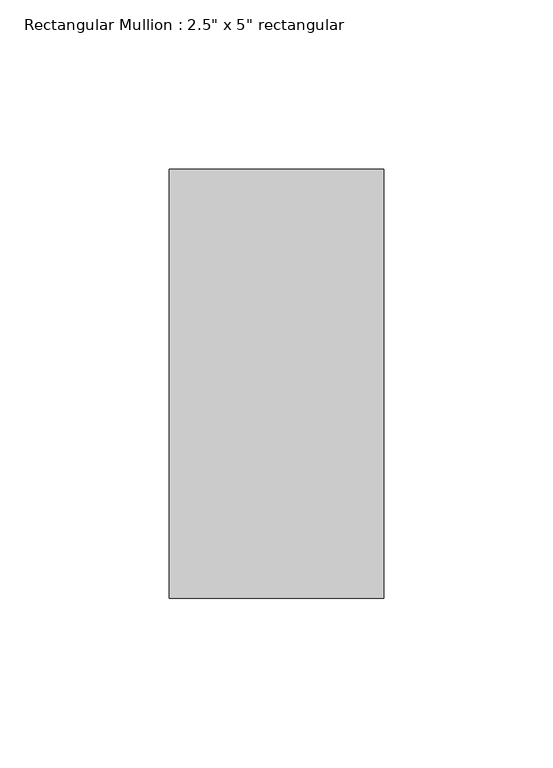
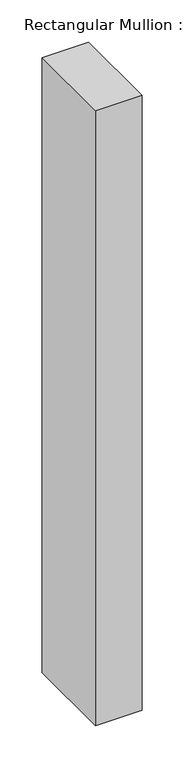
"""IFC4 building model written with IfcOpenShell, lengths in millimetres: member geometry."""

from ifc_helpers import new_model, si_unit, frame, origin, place, context, project, spatial, polyline, outline, extrude, source, transform, mapped, element, save


def member_c067c3a7(model_context):
    return source(origin(), model_context, "Body", "SweptSolid", [
        extrude(outline(polyline([(0.0, 63.5), (0.0, -63.5), (-63.5, -63.5), (-63.5, 63.5), (0.0, 63.5)])), frame((0.0, 0.0, -889.6989237), z_axis=(0.0, 0.0, 1.0), x_axis=(1.0, 0.0, 0.0)), (0.0, 0.0, 1.0), 889.6989237),
    ])


if __name__ == "__main__":
    model = new_model("IFC4")
    model_context = context("Model", 3, world=origin())
    ifc_project = project(units=[si_unit("LENGTHUNIT", "METRE", prefix="MILLI")], contexts=[model_context])
    site = spatial("IfcSite", under=ifc_project)
    building = spatial("IfcBuilding", under=site)
    placement = place(None, origin())
    member_shape = member_c067c3a7(model_context)
    element("IfcMember", 1, ObjectType="Rectangular Mullion : 2.5\" x 5\" rectangular", at=placement, inside=building, context=model_context, shape_type="MappedRepresentation", body=[
        mapped(member_shape, transform((0.0, 0.0, 0.0), x_axis=(1.0, 0.0, 0.0), y_axis=(0.0, 1.0, 0.0), z_axis=(0.0, 0.0, 1.0))),
    ])
    save(model, "model.ifc")

# Revit data of these elements
# Type "Rectangular Mullion : 2.5\" x 5\" rectangular"
#   built-in parameter 1007304 = 0.416667 (stored number, unit not read)
#   built-in parameter 1007301 = 0.104167 (stored number, unit not read)
#   built-in parameter 1007300 = 0.104167 (stored number, unit not read)
# Element 1 (IfcMember, "Rectangular Mullion : 2.5\" x 5\" rectangular")
#   Materials on its faces: "Aluminum"
# Materials
#   "Aluminum": class "Metal", colour RGB 247 247 247, transparency 0, Description = "Aluminum 6061", Cost = 0
